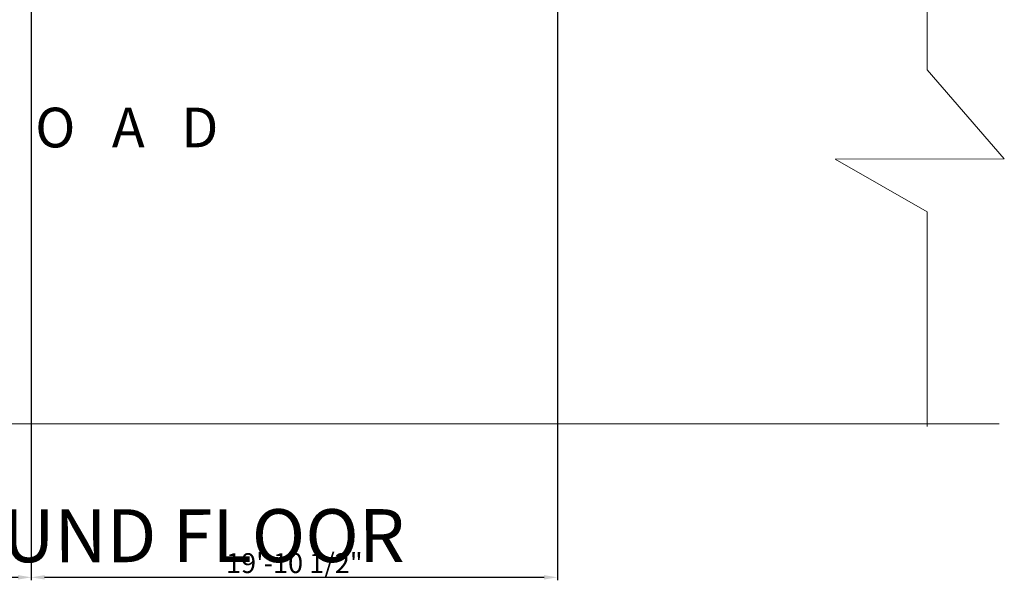
# Model space of a CAD drawing. Units: millimetres. Extents: x 595116 to 630915, y 909473 to 920225.
# Tile 9 of 134: x 629500 to 629946, y 918824 to 919085. Entities that reach past the tile are written whole.
import ezdxf

# ---------------------------------------------------------------- set-up
doc = ezdxf.new("R2010")
doc.units = ezdxf.units.MM
for name, color, linetype, lineweight in [('A-ANNO-TITL', 7, 'Continuous', 35), ('C-ROAD', 30, 'Continuous', 18), ('Dimension', 3, 'Continuous', 18), ('Text', 7, 'Continuous', 18)]:
    doc.layers.add(name, color=color, linetype=linetype, lineweight=lineweight)
doc.styles.get("Standard").update_dxf_attribs({"font": 'arial.ttf'})
doc.dimstyles.new('ISO-25', dxfattribs={"dimtxt": 9, "dimasz": 6, "dimexe": 1.25, "dimexo": 0.625, "dimtad": 1, "dimlunit": 4, "dimtxsty": 'Standard', "dimcen": 2.5, "dimadec": 0, "dimazin": 0, "dimtfac": 1, "dimtmove": 0, "dimatfit": 3, "dimfxl": 1, "dimarcsym": 0})

# ---------------------------------------------------------------- blocks, each defined once
blk = doc.blocks.new('*D215')
at = {"layer": 'Defpoints', "color": 0, "transparency": 16777216}
for p in [(629316.04, 919411.83), (629505.04, 919411.83), (629505.04, 918832.38)]:
    blk.add_point(p, dxfattribs=at)
at = {"layer": 'Dimension', "color": 0, "lineweight": -2, "transparency": 16777216}
for p, q in [((629316.04, 919411.2), (629316.04, 918831.13)), ((629505.04, 919411.2), (629505.04, 918831.13)), ((629322.04, 918832.38), (629499.04, 918832.38))]:
    blk.add_line(p, q, dxfattribs=at)
at = {"layer": 'Dimension', "color": 0, "transparency": 16777216}
for points in [[(629322.04, 918833.38), (629322.04, 918831.38), (629316.04, 918832.38)], [(629499.04, 918833.38), (629499.04, 918831.38), (629505.04, 918832.38)]]:
    blk.add_solid(points, dxfattribs=at)
at = {"layer": 'Dimension', "color": 0, "transparency": 16777216, "insert": (629410.54, 918837.6), "char_height": 9, "attachment_point": 5}
blk.add_mtext('15\'-9"', dxfattribs=at)
blk = doc.blocks.new('*D216')
at = {"layer": 'Defpoints', "color": 0, "transparency": 16777216}
for p in [(629505.04, 919411.83), (629743.54, 919411.93), (629743.54, 918832.38)]:
    blk.add_point(p, dxfattribs=at)
at = {"layer": 'Dimension', "color": 0, "lineweight": -2, "transparency": 16777216}
for p, q in [((629505.04, 919411.2), (629505.04, 918831.13)), ((629743.54, 919411.3), (629743.54, 918831.13)), ((629511.04, 918832.38), (629737.54, 918832.38))]:
    blk.add_line(p, q, dxfattribs=at)
at = {"layer": 'Dimension', "color": 0, "transparency": 16777216}
for points in [[(629511.04, 918833.38), (629511.04, 918831.38), (629505.04, 918832.38)], [(629737.54, 918833.38), (629737.54, 918831.38), (629743.54, 918832.38)]]:
    blk.add_solid(points, dxfattribs=at)
at = {"layer": 'Dimension', "color": 0, "transparency": 16777216, "insert": (629624.29, 918837.66), "char_height": 9, "attachment_point": 5}
blk.add_mtext('19\'-10 1/2"', dxfattribs=at)

msp = doc.modelspace()

# ---------------------------------------------------------------- linework, layer by layer
at = {"layer": 'C-ROAD'}
msp.add_line((629225.95, 918901.928), (629943.895, 918901.928), dxfattribs=at)
msp.add_lwpolyline([(629911.25, 919143.178), (629911.25, 919062.342), (629946.162, 919021.992), (629869.502, 919021.872), (629911.25, 918997.995), (629911.25, 918900.678)], dxfattribs=at)

# ---------------------------------------------------------------- texts
at = {"layer": 'A-ANNO-TITL', "insert": (629372.977, 918863.187), "char_height": 24, "attachment_point": 1, "rotation": 0.01833}
msp.add_mtext_dynamic_manual_height_columns('{       GROUND FLOOR}', width=350.55928, gutter_width=12.5, heights=[0], dxfattribs=at)
at = {"layer": 'Text', "insert": (629469.211, 919045.194), "char_height": 18, "attachment_point": 1, "rotation": 0.01833}
msp.add_mtext_dynamic_manual_height_columns('{R    O   A   D}', width=269.48254, gutter_width=12.5, heights=[0], dxfattribs=at)

# ---------------------------------------------------------------- dimensions: what is measured, and where the dimension line sits
at = {"layer": 'Dimension'}
for base, p1, p2, picture, middle in [((629505.041, 918832.378), (629316.041, 919411.828), (629505.041, 919411.828), '*D215', (629410.541, 918837.598)), ((629743.541, 918832.378), (629505.041, 919411.828), (629743.541, 919411.928), '*D216', (629624.291, 918837.656))]:
    dim = msp.add_linear_dim(base=base, p1=p1, p2=p2, dimstyle='ISO-25', override={"dimdec": 1, "dimlfac": 1, "dimrnd": 0, "dimzin": 1, "dimdsep": 46, "dimlunit": 4, "dimfrac": 2}, dxfattribs=at)
    dim.commit()
    dim.dimension.update_dxf_attribs({"geometry": picture, "text_midpoint": middle})

doc.saveas('drawing.dxf')
